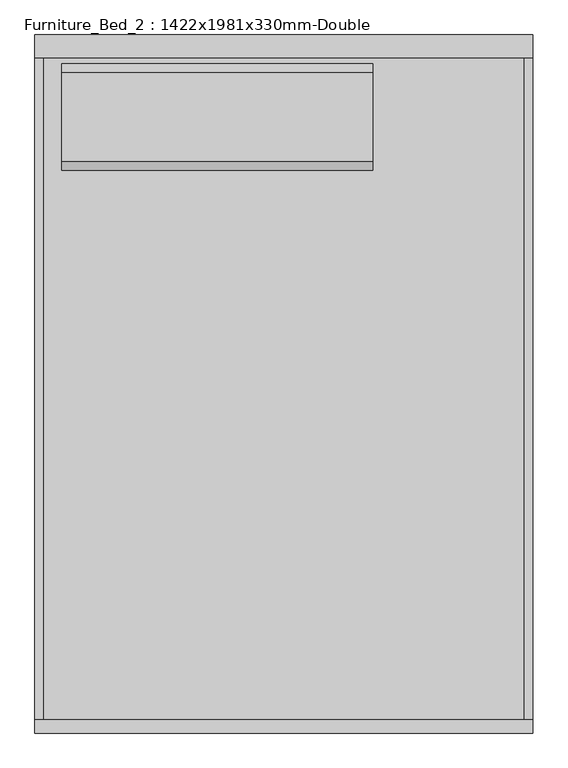
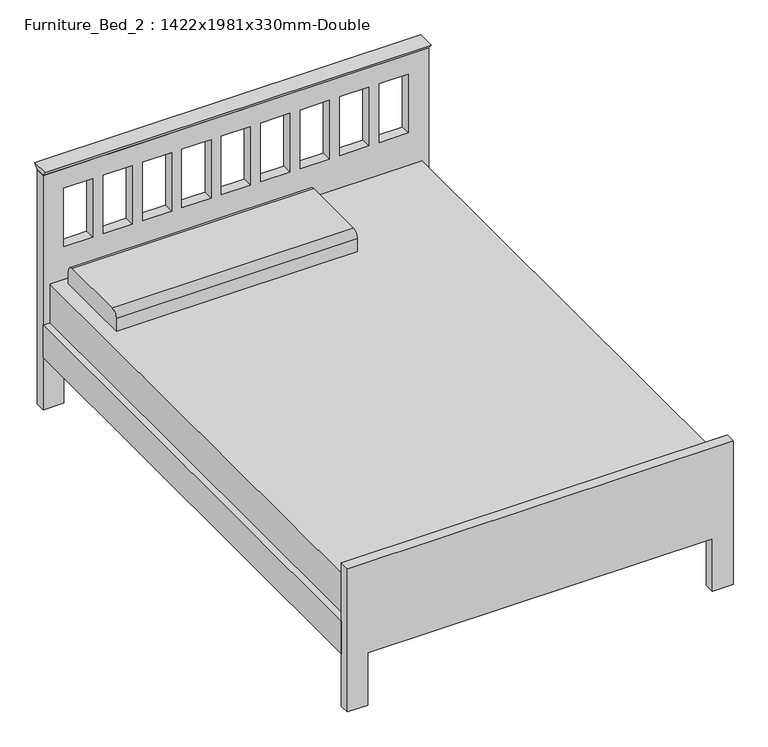
"""IFC4 building model written with IfcOpenShell, lengths in millimetres: furniture geometry, Furniture_Bed_2 : 1422x1981x330mm-Double."""

from ifc_helpers import new_model, si_unit, point, frame, frame_2d, origin, place, context, project, spatial, polyline, circle_curve, trimmed, segment, composite_curve, outline, extrude, source, transform, mapped, element, save


def furniture_bed_2_1422x1981x330mm_double_d56b303b(model_context):
    return source(origin(), model_context, "Body", "SweptSolid", [
        extrude(outline(polyline([(914.4, 692.4168067), (914.4, -730.0365546), (0.0, -730.0365546), (0.0, -654.05), (203.2, -654.05), (203.2, 234.95), (0.0, 234.95), (0.0, 692.4168067), (914.4, 692.4168067)]), holes=[polyline([(838.2, -546.8055556), (609.6, -546.8055556), (609.6, -654.05), (838.2, -654.05), (838.2, -546.8055556)]), polyline([(838.2, -401.4611111), (609.6, -401.4611111), (609.6, -508.7055556), (838.2, -508.7055556), (838.2, -401.4611111)]), polyline([(838.2, -256.1166667), (609.6, -256.1166667), (609.6, -363.3611111), (838.2, -363.3611111), (838.2, -256.1166667)]), polyline([(838.2, -110.7722222), (609.6, -110.7722222), (609.6, -218.0166667), (838.2, -218.0166667), (838.2, -110.7722222)]), polyline([(838.2, 179.9166667), (609.6, 179.9166667), (609.6, 72.6722222), (838.2, 72.6722222), (838.2, 179.9166667)]), polyline([(838.2, 325.2611111), (609.6, 325.2611111), (609.6, 218.0166667), (838.2, 218.0166667), (838.2, 325.2611111)]), polyline([(838.2, 470.6055556), (609.6, 470.6055556), (609.6, 363.3611111), (838.2, 363.3611111), (838.2, 470.6055556)]), polyline([(838.2, 615.95), (609.6, 615.95), (609.6, 508.7055556), (838.2, 508.7055556), (838.2, 615.95)]), polyline([(838.2, 34.5722222), (609.6, 34.5722222), (609.6, -72.6722222), (838.2, -72.6722222), (838.2, 34.5722222)])]), frame((0.0, -38.1, 0.0), z_axis=(0.0, 1.0, 0.0), x_axis=(0.0, 0.0, 1.0)), (0.0, 0.0, 1.0), 38.1),
        extrude(outline(polyline([(0.0, -654.05), (203.2, -654.05), (203.2, 615.95), (0.0, 615.95), (0.0, 692.15), (558.8, 692.15), (558.8, -730.25), (0.0, -730.25), (0.0, -654.05)])), frame((0.0, -1981.2, 0.0), z_axis=(0.0, 1.0, 0.0), x_axis=(0.0, 0.0, 1.0)), (0.0, 0.0, 1.0), 38.1),
        extrude(outline(polyline([(-730.25, -1943.1), (-730.25, -38.1), (-704.85, -38.1), (-704.85, -1943.1), (-730.25, -1943.1)])), frame((0.0, 0.0, 203.5755296), z_axis=(0.0, 0.0, 1.0), x_axis=(1.0, 0.0, 0.0)), (0.0, 0.0, 1.0), 127.0),
        extrude(outline(polyline([(666.75, -1943.1), (666.75, -38.1), (692.15, -38.1), (692.15, -1943.1), (666.75, -1943.1)])), frame((0.0, 0.0, 203.0994861), z_axis=(0.0, 0.0, 1.0), x_axis=(1.0, 0.0, 0.0)), (0.0, 0.0, 1.0), 127.0),
        extrude(outline(polyline([(666.75, -38.1), (666.75, -1943.1), (-704.85, -1943.1), (-704.85, -38.1), (666.75, -38.1)])), frame((0.0, 0.0, 228.6), z_axis=(0.0, 0.0, 1.0), x_axis=(1.0, 0.0, 0.0)), (0.0, 0.0, 1.0), 254.0),
        extrude(outline(composite_curve([segment(polyline([(-373.2486637, 482.6), (-373.2486637, 533.4)]), True, "CONTINUOUS"), segment(trimmed(circle_curve(frame_2d((-347.8486637, 533.4)), 25.4), [point((-373.2486637, 533.4))], [point((-347.8486637, 558.8))], False, "CARTESIAN"), True, "CONTINUOUS"), segment(polyline([(-347.8486637, 558.8), (-93.8486637, 558.8)]), True, "CONTINUOUS"), segment(trimmed(circle_curve(frame_2d((-93.8486637, 533.4)), 25.4), [point((-93.8486637, 558.8))], [point((-68.4486637, 533.4))], False, "CARTESIAN"), True, "CONTINUOUS"), segment(polyline([(-68.4486637, 533.4), (-68.4486637, 482.6), (-373.2486637, 482.6)]), True, "CONTINUOUS")], self_intersect=False)), frame((-654.05, 0.0, 0.0), z_axis=(1.0, 0.0, 0.0), x_axis=(0.0, 1.0, 0.0)), (0.0, 0.0, 1.0), 889.0),
        extrude(outline(polyline([(-38.1, 914.4), (-51.9545455, 933.45), (13.8545455, 933.45), (0.0, 914.4), (-38.1, 914.4)])), frame((-730.0365546, 0.0, 0.0), z_axis=(1.0, 0.0, 0.0), x_axis=(0.0, 1.0, 0.0)), (0.0, 0.0, 1.0), 1422.4533613),
    ])


if __name__ == "__main__":
    model = new_model("IFC4")
    model_context = context("Model", 3, world=origin())
    ifc_project = project(units=[si_unit("LENGTHUNIT", "METRE", prefix="MILLI")], contexts=[model_context])
    site = spatial("IfcSite", under=ifc_project)
    building = spatial("IfcBuilding", under=site)
    placement = place(None, origin())
    furniture_bed_2_1422x1981x330mm_double_shape = furniture_bed_2_1422x1981x330mm_double_d56b303b(model_context)
    element("IfcFurniture", 1, ObjectType="Furniture_Bed_2 : 1422x1981x330mm-Double", at=placement, inside=building, context=model_context, shape_type="MappedRepresentation", body=[
        mapped(furniture_bed_2_1422x1981x330mm_double_shape, transform((0.0, 0.0, 0.0), x_axis=(1.0, 0.0, 0.0), y_axis=(0.0, 1.0, 0.0), z_axis=(0.0, 0.0, 1.0))),
    ])
    save(model, "model.ifc")

# Revit data of these elements
# Type "Furniture_Bed_2 : 1422x1981x330mm-Double"
#   Keynote = "N"
#   Length = 1981.2 mm
#   Width = 1422.4 mm
#   Material Frame = Wood - Birch
#   Material Mattress = Textile - White
#   Default Elevation = 0
# Element 1 (IfcFurniture, "Furniture_Bed_2 : 1422x1981x330mm-Double")
#   Materials on its faces: "Wood - Birch", "Textile - White"
# Materials
#   "Wood - Birch": colour RGB 210 159 95, transparency 0
#   "Textile - White": class "Fabric", colour RGB 247 247 239, transparency 0
